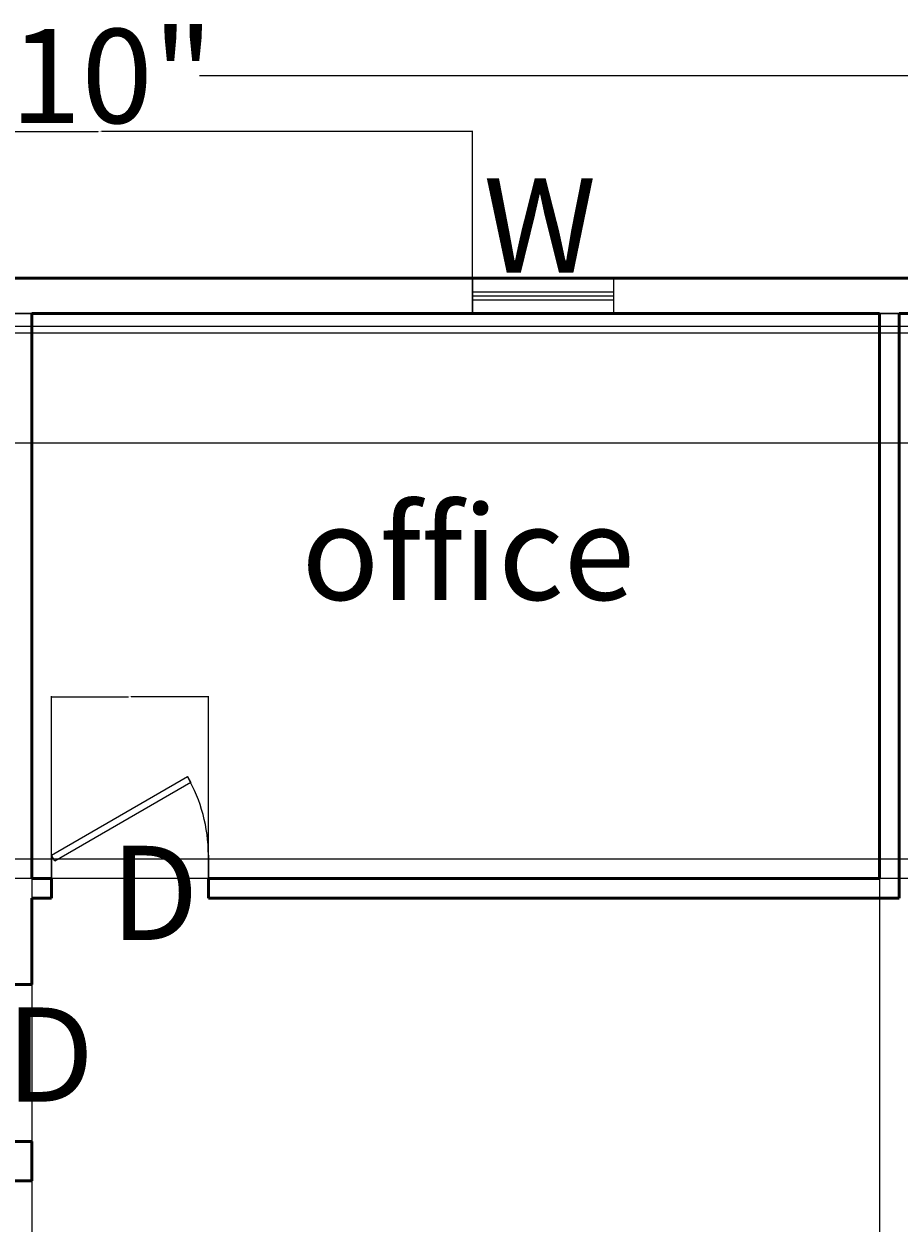
# Model space of a CAD drawing. Units: inches. Extents: x -84 to 931, y 65 to 668.
# Tile 4 of 5: x 426 to 649, y 363 to 668. Entities that reach past the tile are written whole.
import ezdxf

# ---------------------------------------------------------------- set-up
doc = ezdxf.new("R2010")
doc.units = ezdxf.units.IN
doc.header["$MEASUREMENT"] = 0
for name, color, linetype, lineweight in [('A-ANNO-DIMS', 2, 'Continuous', 18), ('A-ANNO-TEXT', 7, 'Continuous', 18), ('A-AREA-IDEN', 7, 'Continuous', 25), ('A-DOOR', 4, 'Continuous', 25), ('A-GLAZ', 4, 'Continuous', 18), ('A-WALL', 7, 'Continuous', 50)]:
    doc.layers.add(name, color=color, linetype=linetype, lineweight=lineweight)
doc.styles.get("Standard").update_dxf_attribs({"font": 'arial.ttf'})
doc.dimstyles.get("Standard").update_dxf_attribs({"dimtxt": 0.18, "dimasz": 0.18, "dimexe": 0.18, "dimexo": 0.0625, "dimgap": 0.09, "dimtad": 0, "dimtih": 1, "dimtoh": 1, "dimdec": 0, "dimzin": 0, "dimdsep": 46, "dimlunit": 3, "dimtxsty": 'Standard', "dimcen": 0.09, "dimadec": 0, "dimazin": 0, "dimtfac": 1, "dimtdec": 0, "dimtofl": 0, "dimtmove": 0, "dimatfit": 3, "dimfxl": 1, "dimtolj": 1, "dimtzin": 0, "dimarcsym": 0})

# ---------------------------------------------------------------- blocks, each defined once
blk = doc.blocks.new('*U4')
for p, q in [((0, 0), (0, -6)), ((40, 0), (40, -6))]:
    blk.add_line(p, q)
blk.add_lwpolyline([(0, 0), (34.64, 20), (35.52, 18.48), (0.87, -1.52)], close=True)
blk.add_arc((0, 0), 40, 0, 30)
blk = doc.blocks.new('*D17')
at = {"layer": 'A-ANNO-DIMS', "color": 0, "lineweight": -2, "transparency": 16777216}
for p, q in [((0.53, 603.58), (0.53, 655.22)), ((0.71, 655.04), (368.83, 655.04)), ((838.35, 655.04), (470.23, 655.04)), ((838.53, 603.58), (838.53, 655.22))]:
    blk.add_line(p, q, dxfattribs=at)
at = {"layer": 'A-ANNO-DIMS', "color": 0, "transparency": 16777216}
for points in [[(0.71, 655.07), (0.71, 655.01), (0.53, 655.04)], [(838.35, 655.07), (838.35, 655.01), (838.53, 655.04)]]:
    blk.add_solid(points, dxfattribs=at)
at = {"layer": 'Defpoints', "color": 0, "transparency": 16777216}
for p in [(838.53, 655.04), (0.53, 603.52), (838.53, 603.52)]:
    blk.add_point(p, dxfattribs=at)
at = {"layer": 'A-ANNO-DIMS', "color": 0, "transparency": 16777216, "insert": (419.53, 655.04), "char_height": 0.18, "attachment_point": 5}
blk.add_mtext('\\A1;{\\H133.33333x;69\'-10"}', dxfattribs=at)
blk = doc.blocks.new('WIN-36IN')
for p, q in [((3.5, 0), (3.5, 36)), ((4.5, 0), (4.5, 36)), ((5.5, 0), (5.5, 36))]:
    blk.add_line(p, q)
blk.add_lwpolyline([(0, 36), (0, 0), (9, 0), (9, 36)], close=True)
blk = doc.blocks.new('*D35')
at = {"layer": 'A-ANNO-DIMS', "color": 0, "lineweight": -2, "transparency": 16777216}
for p, q in [((349.85, 594.58), (349.85, 641.05)), ((350.03, 640.87), (444.4, 640.87)), ((539.69, 640.87), (445.32, 640.87)), ((539.87, 594.58), (539.87, 641.05))]:
    blk.add_line(p, q, dxfattribs=at)
at = {"layer": 'A-ANNO-DIMS', "color": 0, "transparency": 16777216}
for points in [[(350.03, 640.9), (350.03, 640.84), (349.85, 640.87)], [(539.69, 640.9), (539.69, 640.84), (539.87, 640.87)]]:
    blk.add_solid(points, dxfattribs=at)
at = {"layer": 'Defpoints', "color": 0, "transparency": 16777216}
for p in [(539.87, 640.87), (349.85, 594.52), (539.87, 594.52)]:
    blk.add_point(p, dxfattribs=at)
at = {"layer": 'A-ANNO-DIMS', "color": 0, "transparency": 16777216, "insert": (444.86, 640.87), "char_height": 0.18, "attachment_point": 5}
blk.add_mtext('\\A1;15\'-10"', dxfattribs=at)
blk = doc.blocks.new('*D38')
at = {"layer": 'A-ANNO-DIMS', "color": 0, "lineweight": -2, "transparency": 16777216}
for p, q in [((427.53, 594.45), (427.53, 64.99)), ((643.53, 594.45), (643.53, 64.99)), ((427.71, 65.17), (535.14, 65.17)), ((643.35, 65.17), (535.92, 65.17))]:
    blk.add_line(p, q, dxfattribs=at)
at = {"layer": 'A-ANNO-DIMS', "color": 0, "transparency": 16777216}
for points in [[(427.71, 65.2), (427.71, 65.14), (427.53, 65.17)], [(643.35, 65.2), (643.35, 65.14), (643.53, 65.17)]]:
    blk.add_solid(points, dxfattribs=at)
at = {"layer": 'Defpoints', "color": 0, "transparency": 16777216}
for p in [(427.53, 594.52), (643.53, 594.52), (643.53, 65.17)]:
    blk.add_point(p, dxfattribs=at)
at = {"layer": 'A-ANNO-DIMS', "color": 0, "transparency": 16777216, "insert": (535.53, 65.17), "char_height": 0.18, "attachment_point": 5}
blk.add_mtext('\\A1;18\'-0"', dxfattribs=at)
blk = doc.blocks.new('*D55')
at = {"layer": 'A-ANNO-DIMS', "color": 0, "lineweight": -2, "transparency": 16777216}
for p, q in [((704.47, 589.52), (-84, 589.52)), ((-83.82, 589.34), (-83.82, 575.7)), ((-83.82, 561.7), (-83.82, 575.34)), ((704.47, 561.52), (-84, 561.52))]:
    blk.add_line(p, q, dxfattribs=at)
at = {"layer": 'A-ANNO-DIMS', "color": 0, "transparency": 16777216}
for points in [[(-83.85, 589.34), (-83.79, 589.34), (-83.82, 589.52)], [(-83.85, 561.7), (-83.79, 561.7), (-83.82, 561.52)]]:
    blk.add_solid(points, dxfattribs=at)
at = {"layer": 'Defpoints', "color": 0, "transparency": 16777216}
for p in [(-83.82, 589.52), (704.53, 589.52), (704.53, 561.52)]:
    blk.add_point(p, dxfattribs=at)
at = {"layer": 'A-ANNO-DIMS', "color": 0, "transparency": 16777216, "insert": (-83.82, 575.52), "char_height": 0.18, "attachment_point": 5}
blk.add_mtext('\\A1;2\'-4"', dxfattribs=at)
blk = doc.blocks.new('*D62')
at = {"layer": 'A-ANNO-DIMS', "color": 0, "lineweight": -2, "transparency": 16777216}
for p, q in [((643.59, 594.52), (931.06, 594.52)), ((930.88, 594.34), (930.88, 522.7)), ((930.88, 450.7), (930.88, 522.33)), ((829.59, 450.52), (931.06, 450.52))]:
    blk.add_line(p, q, dxfattribs=at)
at = {"layer": 'A-ANNO-DIMS', "color": 0, "transparency": 16777216}
for points in [[(930.85, 594.34), (930.91, 594.34), (930.88, 594.52)], [(930.85, 450.7), (930.91, 450.7), (930.88, 450.52)]]:
    blk.add_solid(points, dxfattribs=at)
at = {"layer": 'Defpoints', "color": 0, "transparency": 16777216}
for p in [(643.53, 594.52), (829.53, 450.52), (930.88, 450.52)]:
    blk.add_point(p, dxfattribs=at)
at = {"layer": 'A-ANNO-DIMS', "color": 0, "transparency": 16777216, "insert": (930.88, 522.52), "char_height": 0.18, "attachment_point": 5}
blk.add_mtext('\\A1;12\'-0"', dxfattribs=at)
blk = doc.blocks.new('*D76')
at = {"layer": 'A-ANNO-DIMS', "color": 0, "lineweight": -2, "transparency": 16777216}
for p, q in [((297.59, 594.52), (931.06, 594.52)), ((930.88, 594.34), (930.88, 593.09)), ((263.98, 591.29), (931.06, 591.29)), ((930.88, 591.47), (930.88, 592.72))]:
    blk.add_line(p, q, dxfattribs=at)
at = {"layer": 'A-ANNO-DIMS', "color": 0, "transparency": 16777216}
for points in [[(930.85, 594.34), (930.91, 594.34), (930.88, 594.52)], [(930.85, 591.47), (930.91, 591.47), (930.88, 591.29)]]:
    blk.add_solid(points, dxfattribs=at)
at = {"layer": 'Defpoints', "color": 0, "transparency": 16777216}
for p in [(297.53, 594.52), (930.88, 594.52), (263.92, 591.29)]:
    blk.add_point(p, dxfattribs=at)
at = {"layer": 'A-ANNO-DIMS', "color": 0, "transparency": 16777216, "insert": (930.88, 592.9), "char_height": 0.18, "attachment_point": 5}
blk.add_mtext('\\A1;0\'-3"', dxfattribs=at)
blk = doc.blocks.new('*D83')
at = {"layer": 'A-ANNO-DIMS', "color": 0, "lineweight": -2, "transparency": 16777216}
for p, q in [((709.47, 594.52), (-84, 594.52)), ((-83.82, 594.34), (-83.82, 592.2)), ((-83.82, 589.7), (-83.82, 591.83)), ((709.47, 589.52), (-84, 589.52))]:
    blk.add_line(p, q, dxfattribs=at)
at = {"layer": 'A-ANNO-DIMS', "color": 0, "transparency": 16777216}
for points in [[(-83.85, 594.34), (-83.79, 594.34), (-83.82, 594.52)], [(-83.85, 589.7), (-83.79, 589.7), (-83.82, 589.52)]]:
    blk.add_solid(points, dxfattribs=at)
at = {"layer": 'Defpoints', "color": 0, "transparency": 16777216}
for p in [(-83.82, 594.52), (709.53, 594.52), (709.53, 589.52)]:
    blk.add_point(p, dxfattribs=at)
at = {"layer": 'A-ANNO-DIMS', "color": 0, "transparency": 16777216, "insert": (-83.82, 592.02), "char_height": 0.18, "attachment_point": 5}
blk.add_mtext('\\A1;0\'-5"', dxfattribs=at)
blk = doc.blocks.new('*D84')
at = {"layer": 'A-ANNO-DIMS', "color": 0, "lineweight": -2, "transparency": 16777216}
for p, q in [((709.47, 455.52), (-84, 455.52)), ((-83.82, 455.34), (-83.82, 453.2)), ((-83.82, 450.7), (-83.82, 452.83)), ((709.47, 450.52), (-84, 450.52))]:
    blk.add_line(p, q, dxfattribs=at)
at = {"layer": 'A-ANNO-DIMS', "color": 0, "transparency": 16777216}
for points in [[(-83.85, 455.34), (-83.79, 455.34), (-83.82, 455.52)], [(-83.85, 450.7), (-83.79, 450.7), (-83.82, 450.52)]]:
    blk.add_solid(points, dxfattribs=at)
at = {"layer": 'Defpoints', "color": 0, "transparency": 16777216}
for p in [(709.53, 455.52), (-83.82, 450.52), (709.53, 450.52)]:
    blk.add_point(p, dxfattribs=at)
at = {"layer": 'A-ANNO-DIMS', "color": 0, "transparency": 16777216, "insert": (-83.82, 453.02), "char_height": 0.18, "attachment_point": 5}
blk.add_mtext('\\A1;0\'-5"', dxfattribs=at)
blk = doc.blocks.new('*D86')
at = {"layer": 'A-ANNO-DIMS', "color": 0, "lineweight": -2, "transparency": 16777216}
for p, q in [((432.53, 450.58), (432.53, 497.05)), ((432.71, 496.87), (452.2, 496.87)), ((472.35, 496.87), (452.86, 496.87)), ((472.53, 450.58), (472.53, 497.05))]:
    blk.add_line(p, q, dxfattribs=at)
at = {"layer": 'A-ANNO-DIMS', "color": 0, "transparency": 16777216}
for points in [[(432.71, 496.9), (432.71, 496.84), (432.53, 496.87)], [(472.35, 496.9), (472.35, 496.84), (472.53, 496.87)]]:
    blk.add_solid(points, dxfattribs=at)
at = {"layer": 'Defpoints', "color": 0, "transparency": 16777216}
for p in [(472.53, 496.87), (432.53, 450.52), (472.53, 450.52)]:
    blk.add_point(p, dxfattribs=at)
at = {"layer": 'A-ANNO-DIMS', "color": 0, "transparency": 16777216, "insert": (452.53, 496.87), "char_height": 0.18, "attachment_point": 5}
blk.add_mtext('\\A1;3\'-4"', dxfattribs=at)

msp = doc.modelspace()

# ---------------------------------------------------------------- linework, layer by layer
at = {"layer": 'A-WALL'}
for p, q in [((672.53, 603.52), (0.53, 603.52)), ((427.53, 594.52), (427.53, 450.52)), ((643.53, 594.52), (427.53, 594.52)), ((643.53, 594.52), (643.53, 450.52)), ((648.53, 594.52), (648.53, 445.52)), ((704.53, 594.52), (648.53, 594.52)), ((432.53, 450.52), (427.53, 450.52)), ((432.53, 450.52), (432.53, 445.52)), ((643.53, 450.52), (472.53, 450.52)), ((472.53, 450.52), (472.53, 445.52)), ((427.53, 445.52), (427.53, 423.52)), ((432.53, 445.52), (427.53, 445.52)), ((648.53, 445.52), (472.53, 445.52)), ((422.53, 423.52), (427.53, 423.52)), ((422.53, 383.52), (427.53, 383.52)), ((427.53, 383.52), (427.53, 373.52)), ((427.53, 373.52), (292.53, 373.52))]:
    msp.add_line(p, q, dxfattribs=at)

# ---------------------------------------------------------------- block references
at = {"layer": 'A-DOOR'}
msp.add_blockref('*U4', (432.53, 456.52), dxfattribs=at)
at = {"layer": 'A-GLAZ', "rotation": 269.9999999999999}
msp.add_blockref('WIN-36IN', (539.87, 603.52), dxfattribs=at)

# ---------------------------------------------------------------- texts
at = {"layer": 'A-ANNO-TEXT', "char_height": 24, "attachment_point": 1}
for s, width, insert in [('W', 20.4711, (542.63, 628.94)), ('D', 21.9508, (447.51, 458.88)), ('D', 21.9508, (420.9, 417.69))]:
    msp.add_mtext_dynamic_manual_height_columns(s, width=width, gutter_width=1, heights=[0], dxfattribs=dict(at, insert=insert))
at = {"layer": 'A-AREA-IDEN', "insert": (496.24, 545.54), "char_height": 24, "attachment_point": 1}
msp.add_mtext_dynamic_manual_height_columns('office', width=70.4822, gutter_width=1, heights=[0], dxfattribs=at)

# ---------------------------------------------------------------- dimensions: what is measured, and where the dimension line sits
at = {"layer": 'A-ANNO-DIMS'}
dim = msp.add_linear_dim(base=(838.53, 655.04), p1=(0.53, 603.52), p2=(838.53, 603.52), text='{\\H133.33333x;<>}', dimstyle='Standard', override={"dimclrd": 0, "dimclre": 0, "dimclrt": 0}, dxfattribs=at)
dim.commit()
dim.dimension.update_dxf_attribs({"geometry": '*D17', "text_midpoint": (419.53, 655.04)})
for base, p1, p2, picture, middle in [((539.87, 640.87), (349.85, 594.52), (539.87, 594.52), '*D35', (444.86, 640.87)), ((643.53, 65.17), (427.53, 594.52), (643.53, 594.52), '*D38', (535.53, 65.17)), ((472.53, 496.87), (432.53, 450.52), (472.53, 450.52), '*D86', (452.53, 496.87))]:
    dim = msp.add_linear_dim(base=base, p1=p1, p2=p2, dimstyle='Standard', override={"dimdec": 1, "dimlfac": 1, "dimrnd": 0, "dimzin": 1, "dimdsep": 46, "dimlunit": 4, "dimfrac": 2}, dxfattribs=at)
    dim.commit()
    dim.dimension.update_dxf_attribs({"geometry": picture, "text_midpoint": middle})
for base, p1, p2, picture, middle in [((-83.82, 594.52), (709.53, 589.52), (709.53, 594.52), '*D83', (-83.82, 592.02)), ((930.88, 594.52), (263.92, 591.29), (297.53, 594.52), '*D76', (930.88, 592.9)), ((930.88, 450.52), (643.53, 594.52), (829.53, 450.52), '*D62', (930.88, 522.52)), ((-83.82, 589.52), (704.53, 561.52), (704.53, 589.52), '*D55', (-83.82, 575.52)), ((-83.82, 450.52), (709.53, 455.52), (709.53, 450.52), '*D84', (-83.82, 453.02))]:
    dim = msp.add_linear_dim(base=base, p1=p1, p2=p2, angle=90, dimstyle='Standard', override={"dimdec": 1, "dimlfac": 1, "dimrnd": 0, "dimzin": 1, "dimdsep": 46, "dimlunit": 4, "dimfrac": 2}, dxfattribs=at)
    dim.commit()
    dim.dimension.update_dxf_attribs({"geometry": picture, "text_midpoint": middle})

doc.saveas('drawing.dxf')
